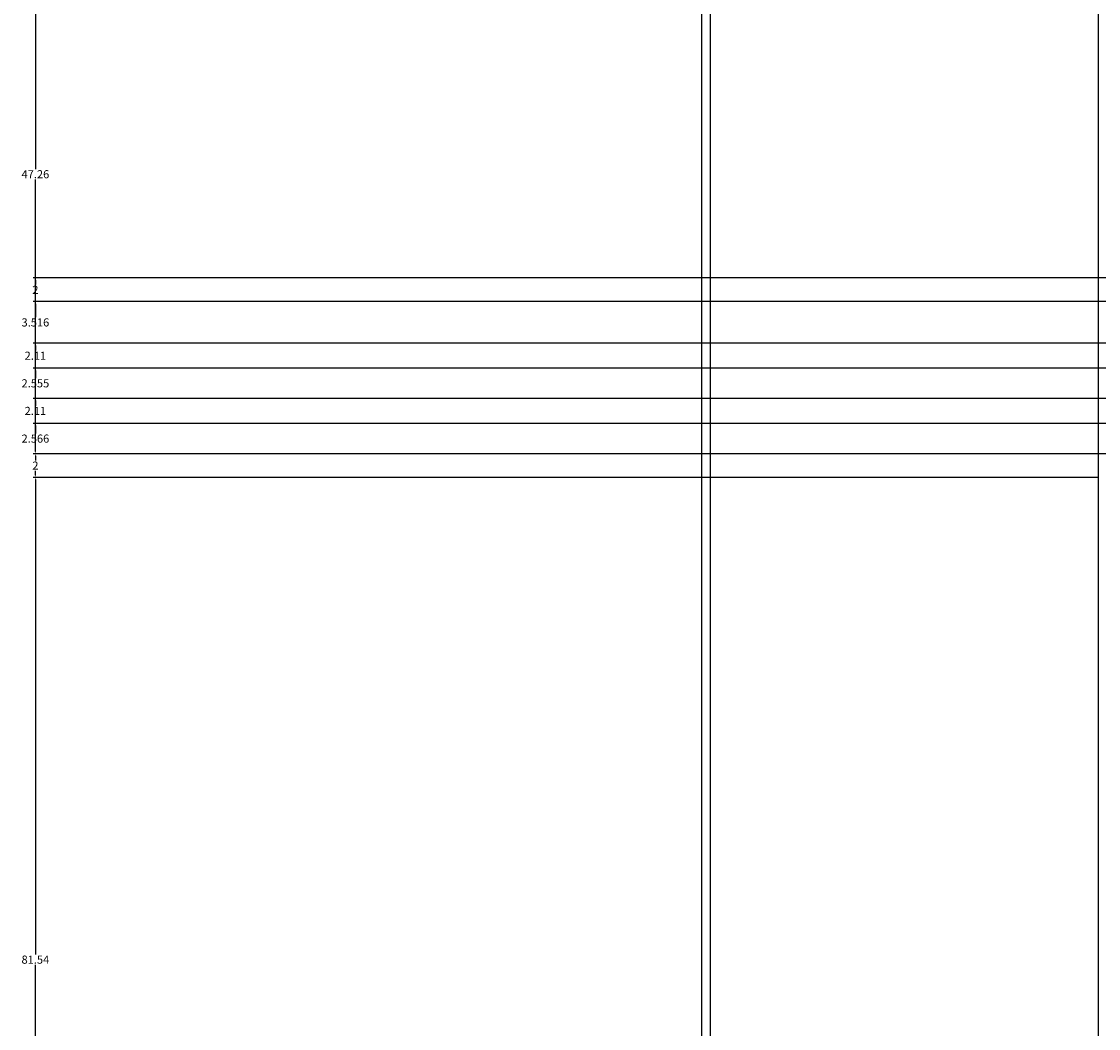
# Model space of a CAD drawing. Units: inches. Extents: x -139 to 346, y 72 to 413.
# Tile 5 of 18: x -138 to -47, y 242 to 328. Entities that reach past the tile are written whole.
import ezdxf

# ---------------------------------------------------------------- set-up
doc = ezdxf.new("R2010")
doc.units = ezdxf.units.IN
doc.header["$MEASUREMENT"] = 0
doc.layers.add('A-ANNO-DIMS', color=2, linetype='Continuous', lineweight=18)
doc.styles.get("Standard").update_dxf_attribs({"font": 'arial.ttf'})
doc.dimstyles.get("Standard").update_dxf_attribs({"dimtxt": 0.6875, "dimasz": 0.18, "dimexe": 0.18, "dimexo": 0.0625, "dimgap": 0.09, "dimtad": 0, "dimtih": 1, "dimtoh": 1, "dimdec": 4, "dimzin": 0, "dimdsep": 46, "dimlunit": 4, "dimtxsty": 'Standard', "dimcen": 0.09, "dimadec": 0, "dimazin": 0, "dimtfac": 1, "dimtdec": 4, "dimtofl": 0, "dimtmove": 0, "dimatfit": 3, "dimfxl": 1, "dimtolj": 1, "dimtzin": 0, "dimarcsym": 0})

# ---------------------------------------------------------------- blocks, each defined once
blk = doc.blocks.new('*D42')
at = {"layer": 'A-ANNO-DIMS', "color": 0, "lineweight": -2, "transparency": 16777216}
for p, q in [((-47.336, 289.06), (-137.304, 289.06)), ((-137.124, 288.88), (-137.124, 248.733)), ((-137.124, 207.704), (-137.124, 247.851)), ((-47.336, 207.524), (-137.304, 207.524))]:
    blk.add_line(p, q, dxfattribs=at)
at = {"layer": 'A-ANNO-DIMS', "color": 0, "transparency": 16777216}
for points in [[(-137.154, 288.88), (-137.094, 288.88), (-137.124, 289.06)], [(-137.154, 207.704), (-137.094, 207.704), (-137.124, 207.524)]]:
    blk.add_solid(points, dxfattribs=at)
at = {"layer": 'Defpoints', "color": 0, "transparency": 16777216}
for p in [(-137.124, 289.06), (-47.273, 289.06), (-47.273, 207.524)]:
    blk.add_point(p, dxfattribs=at)
at = {"layer": 'A-ANNO-DIMS', "color": 0, "transparency": 16777216, "insert": (-137.124, 248.292), "char_height": 0.6875, "attachment_point": 5}
blk.add_mtext('\\A1;81.54', dxfattribs=at)
blk = doc.blocks.new('*D43')
at = {"layer": 'A-ANNO-DIMS', "color": 0, "lineweight": -2, "transparency": 16777216}
for p, q in [((-47.336, 291.06), (-137.304, 291.06)), ((-137.124, 290.88), (-137.124, 290.496)), ((-137.124, 289.24), (-137.124, 289.625)), ((-47.336, 289.06), (-137.304, 289.06))]:
    blk.add_line(p, q, dxfattribs=at)
at = {"layer": 'A-ANNO-DIMS', "color": 0, "transparency": 16777216}
for points in [[(-137.154, 290.88), (-137.094, 290.88), (-137.124, 291.06)], [(-137.154, 289.24), (-137.094, 289.24), (-137.124, 289.06)]]:
    blk.add_solid(points, dxfattribs=at)
at = {"layer": 'Defpoints', "color": 0, "transparency": 16777216}
for p in [(-137.124, 291.06), (-47.273, 291.06), (-47.273, 289.06)]:
    blk.add_point(p, dxfattribs=at)
at = {"layer": 'A-ANNO-DIMS', "color": 0, "transparency": 16777216, "insert": (-137.124, 290.06), "char_height": 0.6875, "attachment_point": 5}
blk.add_mtext('\\A1;2', dxfattribs=at)
blk = doc.blocks.new('*D44')
at = {"layer": 'A-ANNO-DIMS', "color": 0, "lineweight": -2, "transparency": 16777216}
for p, q in [((5.61, 338.322), (-137.304, 338.322)), ((-137.124, 338.142), (-137.124, 315.132)), ((-137.124, 291.24), (-137.124, 314.25)), ((-47.336, 291.06), (-137.304, 291.06))]:
    blk.add_line(p, q, dxfattribs=at)
at = {"layer": 'A-ANNO-DIMS', "color": 0, "transparency": 16777216}
for points in [[(-137.154, 338.142), (-137.094, 338.142), (-137.124, 338.322)], [(-137.154, 291.24), (-137.094, 291.24), (-137.124, 291.06)]]:
    blk.add_solid(points, dxfattribs=at)
at = {"layer": 'Defpoints', "color": 0, "transparency": 16777216}
for p in [(-137.124, 338.322), (5.673, 338.322), (-47.273, 291.06)]:
    blk.add_point(p, dxfattribs=at)
at = {"layer": 'A-ANNO-DIMS', "color": 0, "transparency": 16777216, "insert": (-137.124, 314.691), "char_height": 0.6875, "attachment_point": 5}
blk.add_mtext('\\A1;47.26', dxfattribs=at)
blk = doc.blocks.new('*D49')
at = {"layer": 'A-ANNO-DIMS', "color": 0, "lineweight": -2, "transparency": 16777216}
for p, q in [((-80.796, 213.573), (-80.796, 412.455)), ((-47.273, 226.669), (-47.273, 412.455)), ((-80.616, 412.275), (-65.281, 412.275)), ((-47.453, 412.275), (-62.789, 412.275))]:
    blk.add_line(p, q, dxfattribs=at)
at = {"layer": 'A-ANNO-DIMS', "color": 0, "transparency": 16777216}
for points in [[(-80.616, 412.305), (-80.616, 412.245), (-80.796, 412.275)], [(-47.453, 412.305), (-47.453, 412.245), (-47.273, 412.275)]]:
    blk.add_solid(points, dxfattribs=at)
at = {"layer": 'Defpoints', "color": 0, "transparency": 16777216}
for p in [(-47.273, 412.275), (-47.273, 226.606), (-80.796, 213.511)]:
    blk.add_point(p, dxfattribs=at)
at = {"layer": 'A-ANNO-DIMS', "color": 0, "transparency": 16777216, "insert": (-64.035, 412.275), "char_height": 0.6875, "attachment_point": 5}
blk.add_mtext('\\A1;33.52', dxfattribs=at)
blk = doc.blocks.new('*D50')
at = {"layer": 'A-ANNO-DIMS', "color": 0, "lineweight": -2, "transparency": 16777216}
for p, q in [((-80.796, 213.573), (-80.796, 412.455)), ((-80.068, 211.71), (-80.068, 412.455)), ((-80.616, 412.275), (-80.248, 412.275)), ((-80.068, 412.275), (-79.888, 412.275))]:
    blk.add_line(p, q, dxfattribs=at)
at = {"layer": 'A-ANNO-DIMS', "color": 0, "transparency": 16777216}
for points in [[(-80.616, 412.305), (-80.616, 412.245), (-80.796, 412.275)], [(-80.248, 412.305), (-80.248, 412.245), (-80.068, 412.275)]]:
    blk.add_solid(points, dxfattribs=at)
at = {"layer": 'Defpoints', "color": 0, "transparency": 16777216}
for p in [(-80.068, 412.275), (-80.796, 213.511), (-80.068, 211.648)]:
    blk.add_point(p, dxfattribs=at)
at = {"layer": 'A-ANNO-DIMS', "color": 0, "transparency": 16777216, "insert": (-78.905, 412.275), "char_height": 0.6875, "attachment_point": 5}
blk.add_mtext('\\A1;0.73', dxfattribs=at)
blk = doc.blocks.new('*D89')
at = {"layer": 'A-ANNO-DIMS', "color": 0, "lineweight": -2, "transparency": 16777216}
for p, q in [((62.363, 338.322), (-137.304, 338.322)), ((-137.124, 338.142), (-137.124, 315.132)), ((-137.124, 291.24), (-137.124, 314.25)), ((62.363, 291.06), (-137.304, 291.06))]:
    blk.add_line(p, q, dxfattribs=at)
at = {"layer": 'A-ANNO-DIMS', "color": 0, "transparency": 16777216}
for points in [[(-137.154, 338.142), (-137.094, 338.142), (-137.124, 338.322)], [(-137.154, 291.24), (-137.094, 291.24), (-137.124, 291.06)]]:
    blk.add_solid(points, dxfattribs=at)
at = {"layer": 'Defpoints', "color": 0, "transparency": 16777216}
for p in [(-137.124, 338.322), (62.426, 338.322), (62.426, 291.06)]:
    blk.add_point(p, dxfattribs=at)
at = {"layer": 'A-ANNO-DIMS', "color": 0, "transparency": 16777216, "insert": (-137.124, 314.691), "char_height": 0.6875, "attachment_point": 5}
blk.add_mtext('\\A1;47.26', dxfattribs=at)
blk = doc.blocks.new('*D95')
at = {"layer": 'A-ANNO-DIMS', "color": 0, "lineweight": -2, "transparency": 16777216}
for p, q in [((98.61, 293.626), (-137.304, 293.626)), ((-137.124, 293.446), (-137.124, 292.784)), ((-137.124, 291.24), (-137.124, 291.902)), ((98.61, 291.06), (-137.304, 291.06))]:
    blk.add_line(p, q, dxfattribs=at)
at = {"layer": 'A-ANNO-DIMS', "color": 0, "transparency": 16777216}
for points in [[(-137.154, 293.446), (-137.094, 293.446), (-137.124, 293.626)], [(-137.154, 291.24), (-137.094, 291.24), (-137.124, 291.06)]]:
    blk.add_solid(points, dxfattribs=at)
at = {"layer": 'Defpoints', "color": 0, "transparency": 16777216}
for p in [(-137.124, 293.626), (98.672, 293.626), (98.672, 291.06)]:
    blk.add_point(p, dxfattribs=at)
at = {"layer": 'A-ANNO-DIMS', "color": 0, "transparency": 16777216, "insert": (-137.124, 292.343), "char_height": 0.6875, "attachment_point": 5}
blk.add_mtext('\\A1;2.566', dxfattribs=at)
blk = doc.blocks.new('*D96')
at = {"layer": 'A-ANNO-DIMS', "color": 0, "lineweight": -2, "transparency": 16777216}
for p, q in [((98.61, 295.738), (-137.304, 295.738)), ((-137.124, 295.558), (-137.124, 295.117)), ((-137.124, 293.806), (-137.124, 294.247)), ((98.61, 293.626), (-137.304, 293.626))]:
    blk.add_line(p, q, dxfattribs=at)
at = {"layer": 'A-ANNO-DIMS', "color": 0, "transparency": 16777216}
for points in [[(-137.154, 295.558), (-137.094, 295.558), (-137.124, 295.738)], [(-137.154, 293.806), (-137.094, 293.806), (-137.124, 293.626)]]:
    blk.add_solid(points, dxfattribs=at)
at = {"layer": 'Defpoints', "color": 0, "transparency": 16777216}
for p in [(-137.124, 295.738), (98.672, 295.738), (98.672, 293.626)]:
    blk.add_point(p, dxfattribs=at)
at = {"layer": 'A-ANNO-DIMS', "color": 0, "transparency": 16777216, "insert": (-137.124, 294.682), "char_height": 0.6875, "attachment_point": 5}
blk.add_mtext('\\A1;2.11', dxfattribs=at)
blk = doc.blocks.new('*D97')
at = {"layer": 'A-ANNO-DIMS', "color": 0, "lineweight": -2, "transparency": 16777216}
for p, q in [((98.61, 298.293), (-137.304, 298.293)), ((-137.124, 298.113), (-137.124, 297.456)), ((-137.124, 295.918), (-137.124, 296.574)), ((98.61, 295.738), (-137.304, 295.738))]:
    blk.add_line(p, q, dxfattribs=at)
at = {"layer": 'A-ANNO-DIMS', "color": 0, "transparency": 16777216}
for points in [[(-137.154, 298.113), (-137.094, 298.113), (-137.124, 298.293)], [(-137.154, 295.918), (-137.094, 295.918), (-137.124, 295.738)]]:
    blk.add_solid(points, dxfattribs=at)
at = {"layer": 'Defpoints', "color": 0, "transparency": 16777216}
for p in [(-137.124, 298.293), (98.672, 298.293), (98.672, 295.738)]:
    blk.add_point(p, dxfattribs=at)
at = {"layer": 'A-ANNO-DIMS', "color": 0, "transparency": 16777216, "insert": (-137.124, 297.015), "char_height": 0.6875, "attachment_point": 5}
blk.add_mtext('\\A1;2.555', dxfattribs=at)
blk = doc.blocks.new('*D98')
at = {"layer": 'A-ANNO-DIMS', "color": 0, "lineweight": -2, "transparency": 16777216}
for p, q in [((98.61, 300.405), (-137.304, 300.405)), ((-137.124, 300.225), (-137.124, 299.784)), ((-137.124, 298.473), (-137.124, 298.914)), ((98.61, 298.293), (-137.304, 298.293))]:
    blk.add_line(p, q, dxfattribs=at)
at = {"layer": 'A-ANNO-DIMS', "color": 0, "transparency": 16777216}
for points in [[(-137.154, 300.225), (-137.094, 300.225), (-137.124, 300.405)], [(-137.154, 298.473), (-137.094, 298.473), (-137.124, 298.293)]]:
    blk.add_solid(points, dxfattribs=at)
at = {"layer": 'Defpoints', "color": 0, "transparency": 16777216}
for p in [(-137.124, 300.405), (98.672, 300.405), (98.672, 298.293)]:
    blk.add_point(p, dxfattribs=at)
at = {"layer": 'A-ANNO-DIMS', "color": 0, "transparency": 16777216, "insert": (-137.124, 299.349), "char_height": 0.6875, "attachment_point": 5}
blk.add_mtext('\\A1;2.11', dxfattribs=at)
blk = doc.blocks.new('*D99')
at = {"layer": 'A-ANNO-DIMS', "color": 0, "lineweight": -2, "transparency": 16777216}
for p, q in [((98.61, 303.921), (-137.304, 303.921)), ((-137.124, 303.741), (-137.124, 302.604)), ((-137.124, 300.585), (-137.124, 301.721)), ((98.61, 300.405), (-137.304, 300.405))]:
    blk.add_line(p, q, dxfattribs=at)
at = {"layer": 'A-ANNO-DIMS', "color": 0, "transparency": 16777216}
for points in [[(-137.154, 303.741), (-137.094, 303.741), (-137.124, 303.921)], [(-137.154, 300.585), (-137.094, 300.585), (-137.124, 300.405)]]:
    blk.add_solid(points, dxfattribs=at)
at = {"layer": 'Defpoints', "color": 0, "transparency": 16777216}
for p in [(-137.124, 303.921), (98.672, 303.921), (98.672, 300.405)]:
    blk.add_point(p, dxfattribs=at)
at = {"layer": 'A-ANNO-DIMS', "color": 0, "transparency": 16777216, "insert": (-137.124, 302.163), "char_height": 0.6875, "attachment_point": 5}
blk.add_mtext('\\A1;3.516', dxfattribs=at)
blk = doc.blocks.new('*D100')
at = {"layer": 'A-ANNO-DIMS', "color": 0, "lineweight": -2, "transparency": 16777216}
for p, q in [((98.61, 305.921), (-137.304, 305.921)), ((-137.124, 305.741), (-137.124, 305.356)), ((-137.124, 304.101), (-137.124, 304.485)), ((98.61, 303.921), (-137.304, 303.921))]:
    blk.add_line(p, q, dxfattribs=at)
at = {"layer": 'A-ANNO-DIMS', "color": 0, "transparency": 16777216}
for points in [[(-137.154, 305.741), (-137.094, 305.741), (-137.124, 305.921)], [(-137.154, 304.101), (-137.094, 304.101), (-137.124, 303.921)]]:
    blk.add_solid(points, dxfattribs=at)
at = {"layer": 'Defpoints', "color": 0, "transparency": 16777216}
for p in [(-137.124, 305.921), (98.672, 305.921), (98.672, 303.921)]:
    blk.add_point(p, dxfattribs=at)
at = {"layer": 'A-ANNO-DIMS', "color": 0, "transparency": 16777216, "insert": (-137.124, 304.921), "char_height": 0.6875, "attachment_point": 5}
blk.add_mtext('\\A1;2', dxfattribs=at)

msp = doc.modelspace()

# ---------------------------------------------------------------- dimensions: what is measured, and where the dimension line sits
at = {"layer": 'A-ANNO-DIMS'}
for base, p2, picture, middle in [((-47.2734, 412.2748), (-47.2734, 226.6062), '*D49', (-64.0348, 412.2748)), ((-80.0684, 412.2748), (-80.0684, 211.6478), '*D50', (-78.9055, 412.2748))]:
    dim = msp.add_linear_dim(base=base, p1=(-80.7961, 213.5107), p2=p2, dimstyle='Standard', override={"dimdec": 2, "dimlfac": 1, "dimrnd": 0, "dimzin": 0, "dimdsep": 46, "dimlunit": 2}, dxfattribs=at)
    dim.commit()
    dim.dimension.update_dxf_attribs({"geometry": picture, "text_midpoint": middle})
for base, p1, p2, override, picture, middle in [((-137.1237, 338.3217), (-47.2734, 291.0604), (5.6729, 338.3217), {"dimdec": 2, "dimlfac": 1, "dimrnd": 0, "dimzin": 0, "dimdsep": 46, "dimlunit": 2}, '*D44', (-137.1237, 314.691)), ((-137.1237, 338.3217), (62.4258, 291.0604), (62.4258, 338.3217), {"dimdec": 2, "dimlfac": 1, "dimrnd": 0, "dimzin": 0, "dimdsep": 46, "dimlunit": 2}, '*D89', (-137.1237, 314.691)), ((-137.1237, 305.9205), (98.6724, 303.9205), (98.6724, 305.9205), {"dimdec": 0, "dimlfac": 1, "dimrnd": 0, "dimzin": 0, "dimdsep": 46, "dimlunit": 2}, '*D100', (-137.1237, 304.9205)), ((-137.1237, 303.9205), (98.6724, 300.4047), (98.6724, 303.9205), {"dimdec": 3, "dimlfac": 1, "dimrnd": 0, "dimzin": 0, "dimdsep": 46, "dimlunit": 2}, '*D99', (-137.1237, 302.1626)), ((-137.1237, 300.4047), (98.6724, 298.293), (98.6724, 300.4047), {"dimdec": 2, "dimlfac": 1, "dimrnd": 0, "dimzin": 0, "dimdsep": 46, "dimlunit": 2}, '*D98', (-137.1237, 299.3488)), ((-137.1237, 298.293), (98.6724, 295.7379), (98.6724, 298.293), {"dimdec": 3, "dimlfac": 1, "dimrnd": 0, "dimzin": 0, "dimdsep": 46, "dimlunit": 2}, '*D97', (-137.1237, 297.0155)), ((-137.1237, 295.7379), (98.6724, 293.6263), (98.6724, 295.7379), {"dimdec": 2, "dimlfac": 1, "dimrnd": 0, "dimzin": 0, "dimdsep": 46, "dimlunit": 2}, '*D96', (-137.1237, 294.6821)), ((-137.1237, 293.6263), (98.6724, 291.0604), (98.6724, 293.6263), {"dimdec": 3, "dimlfac": 1, "dimrnd": 0, "dimzin": 0, "dimdsep": 46, "dimlunit": 2}, '*D95', (-137.1237, 292.3433)), ((-137.1237, 291.0604), (-47.2734, 289.0604), (-47.2734, 291.0604), {"dimdec": 0, "dimlfac": 1, "dimrnd": 0, "dimzin": 0, "dimdsep": 46, "dimlunit": 2}, '*D43', (-137.1237, 290.0604)), ((-137.1237, 289.0604), (-47.2734, 207.5243), (-47.2734, 289.0604), {"dimdec": 2, "dimlfac": 1, "dimrnd": 0, "dimzin": 0, "dimdsep": 46, "dimlunit": 2}, '*D42', (-137.1237, 248.2924))]:
    dim = msp.add_linear_dim(base=base, p1=p1, p2=p2, angle=90, dimstyle='Standard', override=override, dxfattribs=at)
    dim.commit()
    dim.dimension.update_dxf_attribs({"geometry": picture, "text_midpoint": middle})

doc.saveas('drawing.dxf')
